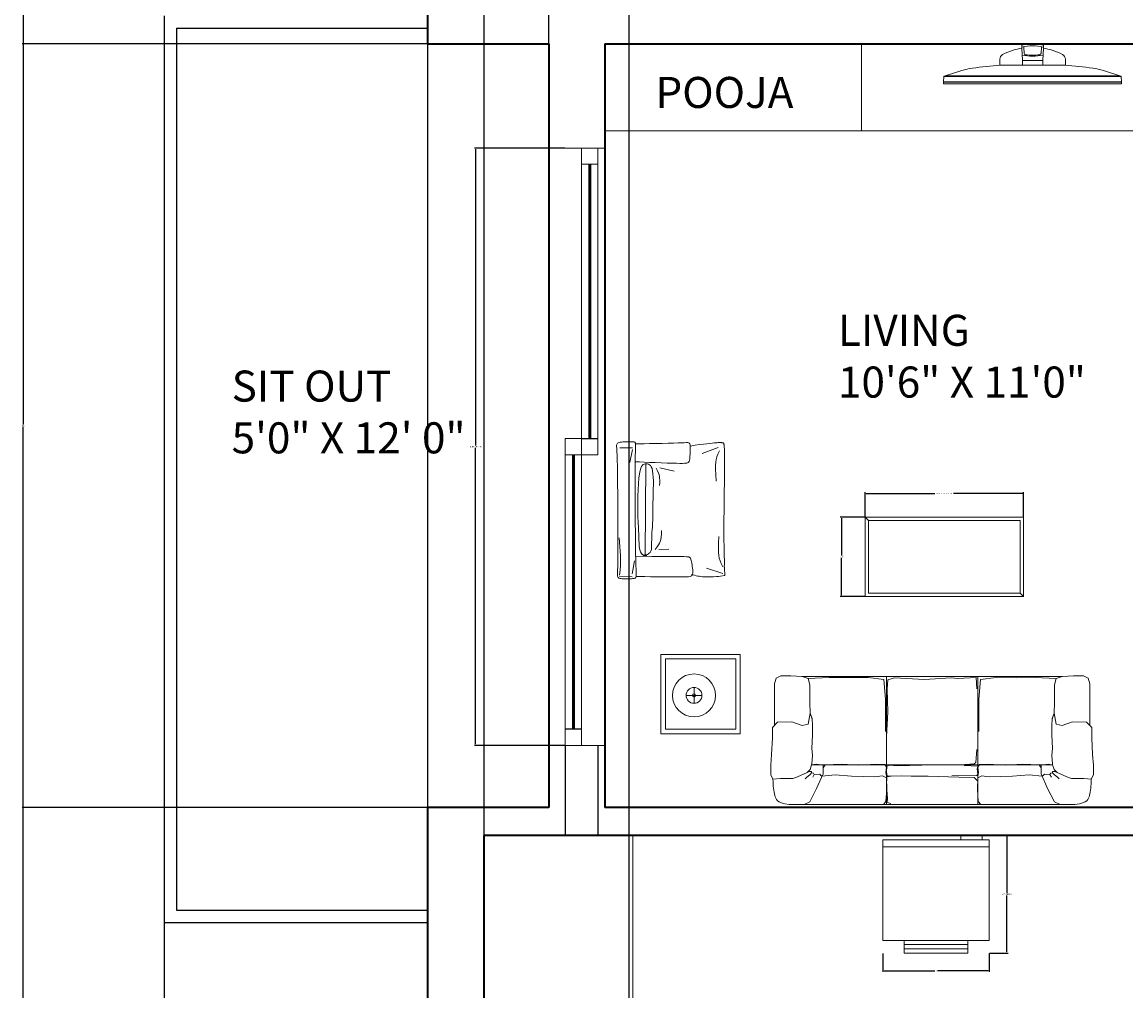
# Model space of a CAD drawing. Units: inches. Extents: x 1723 to 2209, y 1326 to 1810.
# Tile 2 of 6: x 1723 to 1901, y 1477 to 1633. Entities that reach past the tile are written whole.
import ezdxf

# ---------------------------------------------------------------- set-up
doc = ezdxf.new("R2010")
doc.units = ezdxf.units.IN
doc.layers.get('Defpoints').update_dxf_attribs({"color": 255})
for name, color, linetype, lineweight in [('A-ANNO-DIMS', 2, 'Continuous', 18), ('A-AREA-IDEN', 7, 'Continuous', 18), ('A-EQPM', 8, 'Continuous', 13), ('A-FLOR', 7, 'Continuous', 25), ('A-FLOR-CASE', 9, 'Continuous', 18), ('A-FURN', 8, 'Continuous', 13), ('A-WALL', 7, 'Continuous', 35), ('Sliding Door', 3, 'Continuous', 18)]:
    doc.layers.add(name, color=color, linetype=linetype, lineweight=lineweight)
doc.styles.get("Standard").update_dxf_attribs({"font": 'arial.ttf'})
doc.dimstyles.get("Standard").update_dxf_attribs({"dimtxt": 0.18, "dimasz": 0.18, "dimexe": 0.18, "dimexo": 0.0625, "dimgap": 0.09, "dimtad": 0, "dimtih": 1, "dimtoh": 1, "dimdec": 4, "dimzin": 0, "dimdsep": 46, "dimtxsty": 'Standard', "dimcen": 0.09, "dimadec": 0, "dimazin": 0, "dimtfac": 1, "dimtdec": 4, "dimtofl": 0, "dimtmove": 0, "dimatfit": 3, "dimfxl": 1, "dimtolj": 1, "dimtzin": 0, "dimarcsym": 0})

# ---------------------------------------------------------------- blocks, each defined once
blk = doc.blocks.new('A$C15BA614B')
for p, q in [((0, 720), (0, 81)), ((675, 720), (0, 720)), ((495, 747), (495, 720)), ((630, 747), (495, 747)), ((630, 720), (630, 747)), ((675, 81), (675, 720)), ((675, 675), (0, 675)), ((0, 81), (675, 81)), ((135, 81), (135, 0)), ((540, 81), (540, 0)), ((135, 54), (540, 54)), ((135, 27), (540, 27)), ((135, 0), (540, 0))]:
    blk.add_line(p, q)
blk = doc.blocks.new('sofa 053')
at = {"color": 0}
for p, q in [((-919.5, 900), (188.2, 900)), ((-325.8, 0), (-325.8, 900)), ((-317.6, 813.6), (-313, 892.1)), ((-185.2, 885.5), (-313, 892.1)), ((-185.2, 885.5), (-139.6, 891.1)), ((-139.6, 891.1), (48.6, 880)), ((48.6, 880), (260.2, 891.1)), ((188.2, 900), (316.6, 900)), ((260.2, 891.1), (305.9, 877.2)), ((305.9, 877.2), (311.4, 812.2)), ((316.6, 0), (316.6, 900)), ((316.6, 900), (316.6, 0)), ((910.3, 900), (316.6, 900)), ((311.4, 812.2), (305.9, 651.8)), ((305.9, 651.8), (316.6, 476.9)), ((-850.9, 280), (188.2, 280)), ((188.2, 280), (316.6, 280)), ((841.8, 280), (316.6, 280)), ((143.1, 200.9), (209.4, 202.3)), ((209.4, 202.3), (282.4, 200.9)), ((-997.7, 0), (188.2, 0)), ((188.2, 0), (316.6, 0)), ((988.6, 0), (316.6, 0))]:
    blk.add_line(p, q, dxfattribs=at)
for points in [[(-1112.2, 556.2), (-1112.6, 849.1), (-1101.3, 888.6), (-1067.5, 905.5), (-996.9, 905.5), (-917.9, 899.9), (-875.6, 885.8), (-864.3, 840.7), (-864.3, 716.5), (-861.8, 642.8)], [(-875.6, 885.8), (-728.9, 894.2)], [(-598.4, 891.4), (-454.5, 894.2), (-344.5, 880.1), (-333.2, 741.9), (-333.2, 513.4)], [(719.7, 894.2), (445.3, 894.2), (335.3, 880.1), (324, 741.9), (324, 513.4)], [(866.4, 885.8), (719.7, 894.2)], [(1103, 556.2), (1103.5, 849.1), (1092.2, 888.6), (1058.3, 905.5), (987.8, 905.5), (908.8, 899.9), (866.4, 885.8), (855.1, 840.7), (855.1, 716.5), (852.6, 642.8)], [(-983, 183.4), (-1070.3, 183.4), (-1122.9, 178.4), (-1138, 208.8), (-1138, 276.5), (-1132.4, 352.7), (-1126.7, 468.3), (-1126.7, 541.7), (-1090.1, 578.3), (-991.3, 581.1), (-917.9, 555.8), (-875.6, 564.2), (-861.8, 642.8), (-861.8, 642.8), (-847.2, 601.3)], [(-861.8, 642.8), (-847.4, 605.8), (-845.2, 554.1), (-845.2, 488.4), (-849.5, 396.9), (-845.2, 345.2), (-849.5, 285.9), (-850.9, 280)], [(852.6, 642.8), (838.2, 605.8), (836, 554.1), (836, 488.4), (840.3, 396.9), (836, 345.2), (840.3, 285.9), (841.8, 280)], [(973.8, 183.4), (1061.1, 183.4), (1113.7, 178.4), (1128.9, 208.8), (1128.9, 276.5), (1123.2, 352.7), (1117.6, 468.3), (1117.6, 541.7), (1080.9, 578.3), (982.1, 581.1), (908.8, 555.8), (866.4, 564.2), (852.6, 642.8), (852.6, 642.8), (838, 601.3)], [(-317.8, 387.7), (-312.2, 296.4), (-299.8, 286.8), (-201.6, 279.8)], [(-850.9, 280), (-861.2, 247.6), (-882.3, 226.5), (-951.2, 195.1), (-983, 183.4)], [(-850.9, 280), (-819.2, 285), (-771.2, 276.5), (-771.2, 217.3), (-816.3, 112.9), (-864.3, 19.8), (-904, 0)], [(-771.2, 258.8), (-757.1, 279.3), (-639.4, 285.3), (-522.2, 277.6), (-394.4, 284.5), (-336.6, 281.4), (-325.9, 262.4), (-330.5, 225.2), (-325.8, 200)], [(-142.1, 202.3), (-318.5, 205.1), (-326.1, 214.9), (-321.9, 250.4), (-325.4, 270.6), (-229.9, 275.5)], [(67.1, 276.9), (241.3, 272), (295, 278.3), (313.1, 269.2), (315.9, 229.5), (310.3, 202.3), (282.4, 200.9), (313.8, 195.4), (316.6, 133.3), (309.6, 42.1), (311.7, 18.4), (285.9, 5.1)], [(762, 258.8), (747.9, 279.3), (630.3, 285.3), (513.1, 277.6), (385.3, 284.5), (327.4, 281.4), (316.8, 262.4), (321.3, 225.2), (316.6, 200)], [(841.8, 280), (810, 285), (762, 276.5), (762, 217.3), (807.2, 112.9), (855.1, 19.8), (894.8, 0)], [(841.8, 280), (852.1, 247.6), (873.1, 226.5), (942, 195.1), (973.8, 183.4)], [(-997.7, 0), (-1008.3, 1), (-1039.1, 5.9), (-1062.3, 11.8), (-1079.1, 18.7), (-1090.8, 26.4), (-1098.5, 35), (-1103.5, 44.4), (-1107, 54.4), (-1110, 65), (-1112.8, 76.3), (-1115.2, 88.2), (-1117.4, 101), (-1119.2, 114.6), (-1120.7, 129), (-1121.8, 144.4), (-1122.5, 160.9), (-1122.9, 178.4)], [(-882.3, 226.5), (-866.4, 231.7), (-851, 231.7), (-851, 222.6), (-862.2, 212.1), (-886.8, 189.7), (-897.3, 182)], [(-851, 222.6), (-838.4, 221.9), (-832.8, 211.4), (-842.6, 191.8)], [(-832.8, 211.4), (-793.6, 214.2), (-788, 206.5), (-778.7, 200)], [(-778.7, 200), (-686.5, 208.8), (-569.8, 200), (-406.1, 194.5), (-354.2, 201.3), (-325.2, 189.4), (-323.5, 107.7), (-328.6, 20.9), (-346.5, 0.5)], [(-323.7, 167.8), (-300.7, 189.7), (-191.3, 193), (24.3, 200.7), (143.1, 200.9)], [(769.5, 200), (677.4, 208.8), (560.7, 200), (396.9, 194.5), (345, 201.3), (316.1, 189.4), (314.3, 107.7), (319.5, 20.9), (337.3, 0.5)], [(823.7, 211.4), (784.4, 214.2), (778.8, 206.5), (769.5, 200)], [(841.9, 222.6), (829.3, 221.9), (823.7, 211.4), (833.5, 191.8)], [(873.1, 226.5), (857.3, 231.7), (841.9, 231.7), (841.9, 222.6), (853.1, 212.1), (877.6, 189.7), (888.1, 182)], [(988.6, 0), (999.2, 1), (1030, 5.9), (1053.2, 11.8), (1070, 18.7), (1081.6, 26.4), (1089.3, 35), (1094.3, 44.4), (1097.8, 54.4), (1100.9, 65), (1103.6, 76.3), (1106.1, 88.2), (1108.2, 101), (1110, 114.6), (1111.5, 129), (1112.6, 144.4), (1113.3, 160.9), (1113.7, 178.4)]]:
    blk.add_lwpolyline(points, dxfattribs=at)
at = {"color": 0, "flags": 128}
blk.add_lwpolyline([(-728.9, 894.2), (-598.4, 891.4)], dxfattribs=at)
blk = doc.blocks.new('armchair 042')
at = {"color": 0}
for p, q in [((672.7, 1002.5), (673.1, 1009.6)), ((673.1, 1009.6), (673.7, 1013.9)), ((673.7, 1013.9), (674.6, 1017.2)), ((674.6, 1017.2), (675.9, 1020.1)), ((675.9, 1020.1), (677.7, 1022.5)), ((677.7, 1022.5), (680.2, 1024.5)), ((680.2, 1024.5), (683.6, 1026.2)), ((683.6, 1026.2), (688, 1027.5)), ((688, 1027.5), (693.6, 1028.5)), ((693.6, 1028.5), (700.5, 1029.3)), ((700.5, 1029.3), (708.8, 1030)), ((708.8, 1030), (718.2, 1030.4)), ((718.2, 1030.4), (728.4, 1030.7)), ((728.4, 1030.7), (739, 1030.8)), ((739, 1030.8), (749.7, 1030.7)), ((749.7, 1030.7), (760.2, 1030.5)), ((760.2, 1030.5), (770.1, 1030.1)), ((770.1, 1030.1), (779, 1029.6)), ((779, 1029.6), (786.6, 1028.9)), ((786.6, 1028.9), (793.1, 1028)), ((793.1, 1028), (798.5, 1026.7)), ((798.5, 1026.7), (802.9, 1024.9)), ((802.9, 1024.9), (806.4, 1022.6)), ((806.4, 1022.6), (809.2, 1019.5)), ((809.2, 1019.5), (811.3, 1015.7)), ((811.3, 1015.7), (812.8, 1010.9)), ((812.8, 1010.9), (813.9, 1004.9)), ((813.9, 1004.9), (814.6, 996.9)), ((672.5, 990.1), (672.7, 1002.5)), ((672.5, 984.9), (672.5, 990.1)), ((677.3, 823.2), (672.5, 984.9)), ((814.6, 996.9), (812.5, 908.4)), ((573.7, 837.2), (567.5, 829.9)), ((580.3, 842.4), (573.7, 837.2)), ((587.4, 846), (580.3, 842.4)), ((594.9, 848.2), (587.4, 846)), ((599.1, 854), (591.5, 852.6)), ((602.5, 849.6), (594.9, 848.2)), ((606.8, 854.5), (599.1, 854)), ((610.2, 850.1), (602.5, 849.6)), ((614.4, 853.6), (606.8, 854.5)), ((617.8, 849.1), (610.2, 850.1)), ((621.8, 850), (614.4, 853.6)), ((625.2, 845.6), (617.8, 849.1)), ((628.9, 843), (621.8, 850)), ((632.3, 838.5), (625.2, 845.6)), ((638.8, 826.9), (632.3, 838.5)), ((812.5, 908.4), (812.4, 826.8)), ((557.4, 807.7), (553.9, 678.4)), ((562.1, 820.2), (557.4, 807.7)), ((567.5, 829.9), (562.1, 820.2)), ((644.7, 809.8), (638.8, 826.9)), ((649.7, 786.2), (644.7, 809.8)), ((649.7, 786.2), (654.1, 641.6)), ((678.2, 701.5), (677.3, 823.2)), ((812.4, 826.8), (811.1, 761.6)), ((811.1, 761.6), (811.2, 680.2)), ((7.4, 656), (7.5, 675.3)), ((7.5, 675.3), (7.6, 690.1)), ((7.6, 690.1), (7.8, 709)), ((7.8, 709), (7.9, 714.5)), ((7.9, 714.5), (8, 718.1)), ((553.9, 678.4), (551.1, 659.3)), ((679, 583.6), (678.2, 701.5)), ((811.2, 680.2), (811.3, 600.4)), ((6.9, 566.8), (7.1, 601.6)), ((7.1, 601.6), (7.3, 631.6)), ((7.3, 631.6), (7.4, 656)), ((547.8, 611.8), (547, 584.1)), ((549.1, 637), (547.8, 611.8)), ((551.1, 659.3), (549.1, 637)), ((657.1, 602.6), (654.1, 641.6)), ((659, 557.1), (657.1, 602.6)), ((811.3, 600.4), (811.6, 523.4)), ((4.6, 404), (6.7, 527.8)), ((6.7, 527.8), (6.9, 566.8)), ((546.2, 522.8), (545.8, 489.8)), ((546.5, 554.3), (546.2, 522.8)), ((547, 584.1), (546.5, 554.3)), ((660, 507.3), (659, 557.1)), ((660, 455.3), (660, 507.3)), ((679.6, 474.1), (679, 583.6)), ((811.6, 523.4), (811.9, 450)), ((544.6, 421.1), (543.6, 386.4)), ((545.3, 455.8), (544.6, 421.1)), ((545.8, 489.8), (545.3, 455.8)), ((659, 403.2), (660, 455.3)), ((680.1, 377.5), (679.6, 474.1)), ((811.9, 450), (812.4, 381.2)), ((4.3, 316.1), (4.4, 359.1)), ((4.4, 359.1), (4.6, 404)), ((542.8, 352.2), (542.3, 319.3)), ((543.6, 386.4), (542.8, 352.2)), ((654.7, 307), (657.3, 353.1)), ((657.3, 353.1), (659, 403.2)), ((680.4, 297.5), (680.1, 377.5)), ((812.4, 381.2), (812.9, 318)), ((4, 237.4), (4.1, 275.4)), ((4.1, 275.4), (4.3, 316.1)), ((542.3, 319.3), (542.4, 288.3)), ((542.4, 288.3), (543.2, 259.8)), ((543.2, 259.8), (545, 234.5)), ((647.4, 234.9), (651.4, 267.1)), ((651.4, 267.1), (654.7, 307)), ((680.4, 233), (680.4, 297.5)), ((812.9, 318), (813.5, 261.3)), ((813.5, 261.3), (814.1, 212)), ((3.7, 145), (3.8, 171.8)), ((3.8, 171.8), (3.9, 202.7)), ((3.9, 202.7), (4, 237.4)), ((545, 234.5), (548, 213)), ((548, 213), (552.3, 195.8)), ((552.3, 195.8), (557.9, 182.6)), ((557.9, 182.6), (564.4, 172.9)), ((564.4, 172.9), (571.6, 166.2)), ((618.7, 164), (625.5, 169.4)), ((625.5, 169.4), (631.8, 178.2)), ((631.8, 178.2), (637.6, 191.4)), ((637.6, 191.4), (642.8, 210)), ((642.8, 210), (647.4, 234.9)), ((680.1, 142.7), (680.3, 182.1)), ((680.3, 182.1), (680.4, 233)), ((814.1, 212), (814.8, 170.8)), ((814.8, 170.8), (815.5, 137.1)), ((3.6, 122.8), (3.7, 145)), ((3.6, 104.6), (3.6, 122.8)), ((3.6, 89.9), (3.6, 104.6)), ((3.6, 78.1), (3.6, 89.9)), ((571.6, 166.2), (579.4, 162.1)), ((579.4, 162.1), (587.5, 159.9)), ((587.5, 159.9), (595.7, 159.4)), ((595.7, 159.4), (603.7, 159.9)), ((603.7, 159.9), (611.4, 161.2)), ((611.4, 161.2), (618.7, 164)), ((678.8, 73.3), (679.3, 90.3)), ((679.3, 90.3), (679.7, 112.7)), ((679.7, 112.7), (680.1, 142.7)), ((815.5, 137.1), (816.3, 109.9)), ((816.3, 109.9), (817.1, 88.3)), ((817.1, 88.3), (817.8, 71.3)), ((3.6, 68.7), (3.6, 78.1)), ((3.7, 61), (3.6, 68.7)), ((3.9, 54.4), (3.7, 61)), ((4.1, 48.4), (3.9, 54.4)), ((4.3, 42.5), (4.1, 48.4)), ((4.6, 36.7), (4.3, 42.5)), ((5, 31), (4.6, 36.7)), ((5.4, 25.6), (5, 31)), ((5.9, 20.6), (5.4, 25.6)), ((6.4, 16.1), (5.9, 20.6)), ((6.9, 12.1), (6.4, 16.1)), ((7.5, 8.7), (6.9, 12.1)), ((8.1, 6.1), (7.5, 8.7)), ((8.7, 4.2), (8.1, 6.1)), ((9.4, 2.8), (8.7, 4.2)), ((10.1, 1.9), (9.4, 2.8)), ((10.9, 1.3), (10.1, 1.9)), ((11.8, 1), (10.9, 1.3)), ((12.7, 0.8), (11.8, 1)), ((13.8, 0.7), (12.7, 0.8)), ((15, 0.5), (13.8, 0.7)), ((16.4, 0.2), (15, 0.5)), ((17.8, 0), (16.4, 0.2)), ((69.7, 0.1), (59.3, -0.6)), ((82.4, 1.2), (69.7, 0.1)), ((97.7, 2.6), (82.4, 1.2)), ((115.9, 4.5), (97.7, 2.6)), ((137.4, 6.9), (115.9, 4.5)), ((162.6, 10), (137.4, 6.9)), ((191.8, 13.8), (162.6, 10)), ((225.3, 18.6), (191.8, 13.8)), ((263.5, 24.3), (225.3, 18.6)), ((676.8, 20.1), (676.9, 28.1)), ((676.9, 13.3), (676.8, 20.1)), ((676.9, 28.1), (677.3, 37.3)), ((677.3, 7.6), (676.9, 13.3)), ((677.3, 37.3), (677.7, 47.8)), ((678.1, 3), (677.3, 7.6)), ((677.7, 47.8), (678.2, 59.7)), ((679.4, -0.7), (678.1, 3)), ((678.2, 59.7), (678.8, 73.3)), ((796.6, 38.6), (701.3, 38)), ((813.7, 3.1), (808.9, -0.2)), ((817.1, 7.1), (813.7, 3.1)), ((819.2, 11.8), (817.1, 7.1)), ((817.8, 71.3), (818.6, 58)), ((818.6, 58), (819.2, 47.4)), ((819.2, 47.4), (819.9, 38.5)), ((820.3, 17.3), (819.2, 11.8)), ((819.9, 38.5), (820.4, 30.7)), ((820.6, 23.6), (820.3, 17.3)), ((820.4, 30.7), (820.6, 23.6)), ((19.4, -0.3), (17.8, 0)), ((21, -0.6), (19.4, -0.3)), ((22.8, -0.9), (21, -0.6)), ((24.7, -1.2), (22.8, -0.9)), ((26.7, -1.4), (24.7, -1.2)), ((28.9, -1.7), (26.7, -1.4)), ((31.5, -1.8), (28.9, -1.7)), ((34.7, -1.9), (31.5, -1.8)), ((38.8, -1.8), (34.7, -1.9)), ((44.1, -1.6), (38.8, -1.8)), ((50.8, -1.2), (44.1, -1.6)), ((59.3, -0.6), (50.8, -1.2)), ((681.2, -3.5), (679.4, -0.7)), ((683.6, -5.5), (681.2, -3.5)), ((686.7, -6.8), (683.6, -5.5)), ((690.7, -7.5), (686.7, -6.8)), ((695.7, -7.9), (690.7, -7.5)), ((701.7, -8), (695.7, -7.9)), ((709, -7.9), (701.7, -8)), ((717.6, -7.9), (709, -7.9)), ((727.6, -7.9), (717.6, -7.9)), ((738.6, -7.9), (727.6, -7.9)), ((750.2, -7.8), (738.6, -7.9)), ((761.9, -7.6), (750.2, -7.8)), ((773.5, -7.1), (761.9, -7.6)), ((784.4, -6.2), (773.5, -7.1)), ((794.2, -4.8), (784.4, -6.2)), ((802.5, -2.8), (794.2, -4.8)), ((808.9, -0.2), (802.5, -2.8))]:
    blk.add_line(p, q, dxfattribs=at)
for points in [[(673.7, 1013.8), (664.2, 1013.8), (640.7, 1014), (606.1, 1014.2), (563.7, 1014.5), (516.6, 1014.8), (467.8, 1015.2), (420.6, 1015.6), (378, 1016), (342.6, 1016.4), (314.1, 1016.4), (291.8, 1016), (274.9, 1014.7), (262.6, 1012.3), (254.1, 1008.5), (248.7, 1003), (245.5, 995.6), (243.8, 986.1), (243.3, 974.9), (243.8, 962.5), (245.1, 949.4), (247, 936.2), (249.2, 923.3), (251.5, 911.2), (253.7, 900.6), (255.7, 891.7), (257.5, 884.5), (259.4, 878.8), (261.4, 874.3), (263.7, 870.9), (266.5, 868.4), (270, 866.5), (274.3, 865), (280.2, 863.8), (291, 862.8), (310.5, 862.1), (342.6, 861.7), (391.2, 861.7), (460.2, 861.9), (553.4, 862.5), (673.3, 863.5)], [(703.5, 1015.3), (798.9, 1012.7)], [(15.9, 939.3), (27.9, 914.2), (36.8, 893.4), (43.1, 874.3), (47.1, 854.2), (49.1, 830.5), (49.5, 800.4), (48.8, 761.3), (47.1, 710.5)], [(16.5, 991), (139.2, 949.8)], [(684.9, 894.8), (703.3, 993.6)], [(799.2, 1003.9), (794.7, 964.3), (792.3, 926.3), (791.7, 889.9), (792.5, 854.6), (794.2, 820.3), (796.4, 786.7), (798.9, 753.6), (801.1, 720.8)], [(600.2, 159.7), (604.6, 849.6)], [(501.8, 809.3), (426, 805)], [(528.6, 807.4), (514.3, 788.5), (503.5, 773.2), (495.6, 759.9), (490, 746.9), (486.2, 732.5), (483.5, 715.1), (481.5, 693), (479.5, 664.4)], [(41.4, 59.9), (52.5, 85.4), (60.8, 106.5), (66.4, 125.8), (69.7, 146), (71, 169.8), (70.4, 199.8), (68.3, 238.9), (65, 289.7)], [(520, 190.9), (510.9, 212.2), (504.2, 229), (499.4, 243), (496.2, 255.5), (494.5, 268.3), (493.9, 282.7), (494, 300.5), (494.7, 323.1)], [(493, 189.5), (383.5, 215.7)], [(677.3, 8), (668.7, 7.9), (645.8, 7.5), (611.9, 6.9), (570.2, 6.1), (523.8, 5.2), (476, 4.2), (429.9, 3.1), (388.9, 2), (355.3, 0.9), (328.9, 0), (308.8, -0.8), (294, -1.3), (283.6, -1.4), (276.7, -0.9), (272.3, 0), (269.4, 1.7), (267.3, 4.1), (265.7, 7.3), (264.6, 11.3), (263.9, 16.1), (263.5, 21.6), (263.3, 28), (263.3, 35.2), (263.3, 43.1), (263.4, 51.8), (263.6, 61.2), (263.7, 70.8), (263.9, 80.6), (264.2, 90.2), (264.6, 99.5), (265, 108.3), (265.6, 116.2), (266.3, 123.1), (267.2, 129.1), (268.2, 134.2), (269.6, 138.5), (271.3, 142.2), (273.5, 145.3), (276, 147.8), (279.1, 150), (282.9, 151.8), (288.1, 153.3), (295.6, 154.4), (306.3, 155.2), (321.1, 155.6), (340.9, 155.6), (366.5, 155.1), (398.8, 154.3), (438, 153.1), (482, 151.5), (527.7, 149.8), (572.3, 148.1), (612.9, 146.4), (646.6, 145.1), (670.5, 144.1), (680, 143.7)], [(701.2, 49.6), (719.7, 148.3)], [(50.8, 35.6), (172, 80.9)]]:
    blk.add_lwpolyline(points, dxfattribs=at)
for centre, radius, start, end in [((4.2, 1001.7), 3.43, 101.07019, 170.34951), ((159.3, 182.2), 837.5, 96.59178, 100.71955), ((769.8, -30414.4), 31436.5, 91.11446, 91.28806), ((117.9, 570.8), 447.1, 72.48852, 84.80948), ((57, 992.7), 57, 170.34951, 189.46286), ((-256.2, 940.5), 260.5, 0.55092, 9.46286), ((4370.1, 901.7), 4365.9, 179.458, 182.40994)]:
    blk.add_arc(centre, radius, start, end, dxfattribs=at)
blk = doc.blocks.new('B1')
at = {"color": 0}
for points in [[(-73.6, -0.1), (-73.6, 13.1, -0.272026), (-67.3, 23.9, -0.059641), (-43.9, 33.5, -0.024069), (-24.5, 37.9), (-22.7, 10), (-22.7, 0)], [(-24.5, 37.9), (-24.5, 43.2, -0.236854), (-23.9, 44.5, -0.069077), (0, 47.8, -0.069077)], [(-24.5, 37.7), (-24.5, 38.9, -0.236854), (-23.9, 40.2, -0.069077), (0, 43.6, -0.069077)], [(24.5, 37.9), (24.5, 43.2, 0.236854), (23.9, 44.5, 0.069077), (0, 47.8, 0.069077)], [(24.5, 37.7), (24.5, 38.9, 0.236854), (23.9, 40.2, 0.069077), (0, 43.6, 0.069077)], [(73.6, -0.1), (73.6, 13.1, 0.272026), (67.3, 23.9, 0.059641), (43.9, 33.5, 0.024069), (24.5, 37.9), (22.7, 10), (22.7, 0)], [(-200, -38.4), (-200, -37.7), (-199.2, -25.8, -0.303983), (-198.5, -24.8), (-159.1, -12.4, -0.039649), (-135.4, -7, -0.017831), (-72.5, 0), (0, 0)], [(200, -38.4), (200, -37.7), (199.2, -25.8, 0.303983), (198.5, -24.8), (159.1, -12.4, 0.039649), (135.4, -7, 0.017831), (72.5, 0), (0, 0)]]:
    blk.add_lwpolyline(points, format="xyb", dxfattribs=at)
for points in [[(-19.8, 40.1), (-18.9, 26.4)], [(19.8, 40.1), (18.9, 26.4)], [(-22.7, 10), (0, 10)], [(22.7, 10), (0, 10)], [(-196.3, -24.2), (0, -24.2)], [(196.3, -24.2), (0, -24.2)], [(-200, -37.8), (0, -37.8)], [(-200, -41.4), (-200, -38.4), (200, -38.4)], [(-200, -38.4), (0, -38.4)], [(200, -41.4), (200, -38.4), (-200, -38.4)], [(-199.2, -25.8), (0, -25.8)], [(-198.9, -42.4), (0, -42.4)], [(199.2, -25.8), (0, -25.8)], [(200, -37.8), (0, -37.8)], [(200, -38.4), (0, -38.4)], [(198.9, -42.4), (0, -42.4)]]:
    blk.add_lwpolyline(points, dxfattribs=at)
for centre, radius, start, end in [((-15.4, 26.6), 3.53, 183.678, 262.9963), ((15.4, 26.6), 3.53, 277.0037, 356.322), ((0, 150), 130, 259.5789, 270), ((0, 152.2), 130, 262.9963, 270), ((0, 152.2), 130, 270, 277.0037), ((0, 150), 130, 270, 280.4211), ((-198.9, -41.4), 1.06, 180, 270), ((198.9, -41.4), 1.06, 270, 0)]:
    blk.add_arc(centre, radius, start, end, dxfattribs=at)
blk = doc.blocks.new('A$C7a76cbd6')
at = {"layer": 'Sliding Door'}
for p, q in [((540.4, 283.7, 0), (478.3, 283.7, 0)), ((478.3, 283.7, 0), (540.4, 283.7, 0)), ((540.4, 221.5, 0), (540.4, 283.7, 0)), ((540.4, 283.7, 0), (1585.3, 283.7, 0)), ((540.4, 283.7, 0), (540.4, 221.5, 0)), ((1585.3, 256.6, 0), (540.4, 256.6, 0)), ((540.4, 256.6, 0), (540.4, 248.7, 0)), ((540.4, 252.6, 0), (1584.3, 252.6, 0)), ((1584.3, 283.7, 0), (1647.4, 283.7, 0)), ((1584.3, 283.7, 0), (1584.3, 221.5, 0)), ((1647.4, 283.7, 0), (1585.3, 283.7, 0)), ((1585.3, 283.7, 0), (1585.3, 221.5, 0)), ((1585.3, 248.7, 0), (1585.3, 256.6, 0)), ((1647.4, 221.5, 0), (1647.4, 283.7, 0)), ((1647.4, 283.7, 0), (1647.4, 221.5, 0)), ((478.3, 221.5, 0), (540.4, 221.5, 0)), ((478.3, 221.5, 0), (540.4, 221.5, 0)), ((540.4, 248.7, 0), (1585.3, 248.7, 0)), ((1584.3, 221.5, 0), (540.4, 221.5, 0)), ((1646.4, 221.5, 0), (1584.3, 221.5, 0)), ((1584.3, 221.5, 0), (1584.3, 159.4, 0)), ((1584.3, 221.5, 0), (1647.4, 221.5, 0)), ((1584.3, 221.5, 0), (1647.4, 221.5, 0)), ((1584.3, 221.5, 0), (1584.3, 159.4, 0)), ((1585.3, 221.5, 0), (1647.4, 221.5, 0)), ((1646.4, 159.4, 0), (1646.4, 221.5, 0)), ((1647.4, 221.5, 0), (2691.3, 221.5, 0)), ((1647.4, 221.5, 0), (1647.4, 159.4, 0)), ((2690.3, 221.5, 0), (2753.4, 221.5, 0)), ((2690.3, 221.5, 0), (2690.3, 159.4, 0)), ((2753.4, 221.5, 0), (2691.3, 221.5, 0)), ((2691.3, 221.5, 0), (2691.3, 159.4, 0)), ((2691.3, 194.4, 0), (1647.4, 194.4, 0)), ((1647.4, 194.4, 0), (1647.4, 186.5, 0)), ((1647.4, 190.5, 0), (2690.3, 190.5, 0)), ((1647.4, 186.5, 0), (2691.3, 186.5, 0)), ((2691.3, 186.5, 0), (2691.3, 194.4, 0)), ((1584.3, 159.4, 0), (1646.4, 159.4, 0)), ((1584.3, 159.4, 0), (1647.4, 159.4, 0)), ((2691.3, 159.4, 0), (1646.4, 159.4, 0)), ((2690.3, 159.4, 0), (2753.4, 159.4, 0)), ((2691.3, 159.4, 0), (2753.4, 159.4, 0))]:
    blk.add_line(p, q, dxfattribs=at)
blk = doc.blocks.new('TABLE-END-SMALL')
for p, q in [((5.32, 4.88), (5.32, 7.45)), ((6.6, 6.17), (4.03, 6.17))]:
    blk.add_line(p, q)
for points in [[(0, 0), (12.75, 0), (12.75, 12.75), (0, 12.75)], [(0.71, 0.71), (12.04, 0.71), (12.04, 12.04), (0.71, 12.04)]]:
    blk.add_lwpolyline(points, close=True)
for radius in [3.46, 1.28, 0.266]:
    blk.add_circle((5.32, 6.17), radius)
blk = doc.blocks.new('TABLE-COFFEE-RECT')
for p, q in [((0, 0), (0, 12.75)), ((0, 12.75), (0.53, 12.22)), ((0, 12.75), (25.5, 12.75)), ((25.5, 12.75), (25.5, 0)), ((0.53, 0.53), (0.53, 12.22)), ((0.53, 12.22), (24.97, 12.22)), ((24.97, 12.22), (24.97, 0.53)), ((25.5, 0), (0, 0)), ((24.97, 0.53), (0.53, 0.53)), ((24.97, 0.53), (25.5, 0))]:
    blk.add_line(p, q)
blk = doc.blocks.new('*D63')
at = {"layer": 'A-ANNO-DIMS', "color": 0, "lineweight": -2, "transparency": 16777216}
for p, q in [((1810.16, 1612.41), (1795.61, 1612.41)), ((1795.79, 1612.23), (1795.79, 1564.49)), ((1795.79, 1516.38), (1795.79, 1564.12)), ((1810.16, 1516.2), (1795.61, 1516.2))]:
    blk.add_line(p, q, dxfattribs=at)
at = {"layer": 'A-ANNO-DIMS', "color": 0, "transparency": 16777216}
for points in [[(1795.76, 1612.23), (1795.82, 1612.23), (1795.79, 1612.41)], [(1795.76, 1516.38), (1795.82, 1516.38), (1795.79, 1516.2)]]:
    blk.add_solid(points, dxfattribs=at)
at = {"layer": 'Defpoints', "color": 0, "transparency": 16777216}
for p in [(1810.22, 1612.41), (1795.79, 1516.2), (1810.22, 1516.2)]:
    blk.add_point(p, dxfattribs=at)
at = {"layer": 'A-ANNO-DIMS', "color": 0, "transparency": 16777216, "insert": (1795.79, 1564.31), "char_height": 0.18, "attachment_point": 5}
blk.add_mtext('\\A1;SLIDING UNIT 96', dxfattribs=at)
blk = doc.blocks.new('*D64')
at = {"layer": 'A-ANNO-DIMS', "color": 0, "lineweight": -2, "transparency": 16777216}
for p, q in [((1810.22, 1516.14), (1810.22, 1501.59)), ((1815.48, 1516.14), (1815.48, 1501.59)), ((1810.4, 1501.77), (1812.7, 1501.77)), ((1815.3, 1501.77), (1813, 1501.77))]:
    blk.add_line(p, q, dxfattribs=at)
at = {"layer": 'A-ANNO-DIMS', "color": 0, "transparency": 16777216}
for points in [[(1810.4, 1501.8), (1810.4, 1501.74), (1810.22, 1501.77)], [(1815.3, 1501.8), (1815.3, 1501.74), (1815.48, 1501.77)]]:
    blk.add_solid(points, dxfattribs=at)
at = {"layer": 'Defpoints', "color": 0, "transparency": 16777216}
for p in [(1810.22, 1516.2), (1815.48, 1516.2), (1815.48, 1501.77)]:
    blk.add_point(p, dxfattribs=at)
at = {"layer": 'A-ANNO-DIMS', "color": 0, "transparency": 16777216, "insert": (1812.85, 1501.77), "char_height": 0.18, "attachment_point": 5}
blk.add_mtext('\\A1;5', dxfattribs=at)
blk = doc.blocks.new('*D75')
at = {"layer": 'A-ANNO-DIMS', "color": 0, "lineweight": -2, "transparency": 16777216}
for p, q in [((1858.52, 1553.01), (1858.52, 1556.96)), ((1858.7, 1556.78), (1869.77, 1556.78)), ((1883.85, 1556.78), (1872.78, 1556.78)), ((1884.03, 1553.01), (1884.03, 1556.96))]:
    blk.add_line(p, q, dxfattribs=at)
at = {"layer": 'A-ANNO-DIMS', "color": 0, "transparency": 16777216}
for points in [[(1858.7, 1556.81), (1858.7, 1556.75), (1858.52, 1556.78)], [(1883.85, 1556.81), (1883.85, 1556.75), (1884.03, 1556.78)]]:
    blk.add_solid(points, dxfattribs=at)
at = {"layer": 'Defpoints', "color": 0, "transparency": 16777216}
for p in [(1858.52, 1556.78), (1858.52, 1552.95), (1884.03, 1552.95)]:
    blk.add_point(p, dxfattribs=at)
at = {"layer": 'A-ANNO-DIMS', "color": 0, "transparency": 16777216, "insert": (1871.28, 1556.78), "char_height": 0.18, "attachment_point": 5}
blk.add_mtext('\\A1;COFFEE TABLE 26 TYP.', dxfattribs=at)
blk = doc.blocks.new('*D76')
at = {"layer": 'A-ANNO-DIMS', "color": 0, "lineweight": -2, "transparency": 16777216}
for p, q in [((1858.46, 1552.95), (1854.52, 1552.95)), ((1854.7, 1552.77), (1854.7, 1546.76)), ((1854.7, 1540.38), (1854.7, 1546.39)), ((1858.46, 1540.2), (1854.52, 1540.2))]:
    blk.add_line(p, q, dxfattribs=at)
at = {"layer": 'A-ANNO-DIMS', "color": 0, "transparency": 16777216}
for points in [[(1854.67, 1552.77), (1854.73, 1552.77), (1854.7, 1552.95)], [(1854.67, 1540.38), (1854.73, 1540.38), (1854.7, 1540.2)]]:
    blk.add_solid(points, dxfattribs=at)
at = {"layer": 'Defpoints', "color": 0, "transparency": 16777216}
for p in [(1858.52, 1552.95), (1854.7, 1540.2), (1858.52, 1540.2)]:
    blk.add_point(p, dxfattribs=at)
at = {"layer": 'A-ANNO-DIMS', "color": 0, "transparency": 16777216, "insert": (1854.7, 1546.57), "char_height": 0.18, "attachment_point": 5}
blk.add_mtext('\\A1;13 TYP.', dxfattribs=at)
blk = doc.blocks.new('*D87')
at = {"layer": 'A-ANNO-DIMS', "color": 0, "lineweight": -2, "transparency": 16777216}
for p, q in [((1878.58, 1501.69), (1881.54, 1501.69)), ((1881.36, 1501.51), (1881.36, 1492.4)), ((1881.36, 1482.93), (1881.36, 1492.04)), ((1878.58, 1482.75), (1881.54, 1482.75))]:
    blk.add_line(p, q, dxfattribs=at)
at = {"layer": 'A-ANNO-DIMS', "color": 0, "transparency": 16777216}
for points in [[(1881.33, 1501.51), (1881.39, 1501.51), (1881.36, 1501.69)], [(1881.33, 1482.93), (1881.39, 1482.93), (1881.36, 1482.75)]]:
    blk.add_solid(points, dxfattribs=at)
at = {"layer": 'Defpoints', "color": 0, "transparency": 16777216}
for p in [(1878.52, 1501.69), (1881.36, 1501.69), (1878.52, 1482.75)]:
    blk.add_point(p, dxfattribs=at)
at = {"layer": 'A-ANNO-DIMS', "color": 0, "transparency": 16777216, "insert": (1881.36, 1492.22), "char_height": 0.18, "attachment_point": 5}
blk.add_mtext('\\A1;APPLIANCE 19', dxfattribs=at)
blk = doc.blocks.new('*D88')
at = {"layer": 'A-ANNO-DIMS', "color": 0, "lineweight": -2, "transparency": 16777216}
for p, q in [((1861.4, 1482.69), (1861.4, 1479.73)), ((1878.52, 1482.69), (1878.52, 1479.73)), ((1861.58, 1479.91), (1869.75, 1479.91)), ((1878.34, 1479.91), (1870.17, 1479.91))]:
    blk.add_line(p, q, dxfattribs=at)
at = {"layer": 'A-ANNO-DIMS', "color": 0, "transparency": 16777216}
for points in [[(1861.58, 1479.94), (1861.58, 1479.88), (1861.4, 1479.91)], [(1878.34, 1479.94), (1878.34, 1479.88), (1878.52, 1479.91)]]:
    blk.add_solid(points, dxfattribs=at)
at = {"layer": 'Defpoints', "color": 0, "transparency": 16777216}
for p in [(1861.4, 1482.75), (1878.52, 1482.75), (1878.52, 1479.91)]:
    blk.add_point(p, dxfattribs=at)
at = {"layer": 'A-ANNO-DIMS', "color": 0, "transparency": 16777216, "insert": (1869.96, 1479.91), "char_height": 0.18, "attachment_point": 5}
blk.add_mtext('\\A1;17', dxfattribs=at)
blk = doc.blocks.new('*D94')
at = {"layer": 'A-ANNO-DIMS', "color": 0, "lineweight": -2, "transparency": 16777216}
for p, q in [((1788.04, 1786.69), (1722.75, 1786.69)), ((1722.93, 1786.51), (1722.93, 1567.87)), ((1722.93, 1348.87), (1722.93, 1567.51)), ((1788.04, 1348.69), (1722.75, 1348.69))]:
    blk.add_line(p, q, dxfattribs=at)
at = {"layer": 'A-ANNO-DIMS', "color": 0, "transparency": 16777216}
for points in [[(1722.9, 1786.51), (1722.96, 1786.51), (1722.93, 1786.69)], [(1722.9, 1348.87), (1722.96, 1348.87), (1722.93, 1348.69)]]:
    blk.add_solid(points, dxfattribs=at)
at = {"layer": 'Defpoints', "color": 0, "transparency": 16777216}
for p in [(1722.93, 1786.69), (1788.1, 1786.69), (1788.1, 1348.69)]:
    blk.add_point(p, dxfattribs=at)
at = {"layer": 'A-ANNO-DIMS', "color": 0, "transparency": 16777216, "insert": (1722.93, 1567.69), "char_height": 0.18, "attachment_point": 5}
blk.add_mtext('\\A1;438', dxfattribs=at)
blk = doc.blocks.new('*D95')
at = {"layer": 'A-ANNO-DIMS', "color": 0, "lineweight": -2, "transparency": 16777216}
for p, q in [((1745.6, 1487.63), (1745.6, 1325.84)), ((1788.1, 1348.63), (1788.1, 1325.84)), ((1745.78, 1326.02), (1766.53, 1326.02)), ((1787.92, 1326.02), (1767.18, 1326.02))]:
    blk.add_line(p, q, dxfattribs=at)
at = {"layer": 'A-ANNO-DIMS', "color": 0, "transparency": 16777216}
for points in [[(1745.78, 1326.05), (1745.78, 1325.99), (1745.6, 1326.02)], [(1787.92, 1326.05), (1787.92, 1325.99), (1788.1, 1326.02)]]:
    blk.add_solid(points, dxfattribs=at)
at = {"layer": 'Defpoints', "color": 0, "transparency": 16777216}
for p in [(1745.6, 1487.69), (1788.1, 1348.69), (1788.1, 1326.02)]:
    blk.add_point(p, dxfattribs=at)
at = {"layer": 'A-ANNO-DIMS', "color": 0, "transparency": 16777216, "insert": (1766.85, 1326.02), "char_height": 0.18, "attachment_point": 5}
blk.add_mtext('\\A1;42.5', dxfattribs=at)
blk = doc.blocks.new('*D110')
at = {"layer": 'A-ANNO-DIMS', "color": 0, "lineweight": -2, "transparency": 16777216}
for p, q in [((1788.1, 1506.25), (1788.1, 1809.54)), ((1788.28, 1809.36), (1797.54, 1809.36)), ((1807.42, 1809.36), (1798.17, 1809.36)), ((1807.6, 1506.25), (1807.6, 1809.54))]:
    blk.add_line(p, q, dxfattribs=at)
at = {"layer": 'A-ANNO-DIMS', "color": 0, "transparency": 16777216}
for points in [[(1788.28, 1809.39), (1788.28, 1809.33), (1788.1, 1809.36)], [(1807.42, 1809.39), (1807.42, 1809.33), (1807.6, 1809.36)]]:
    blk.add_solid(points, dxfattribs=at)
at = {"layer": 'Defpoints', "color": 0, "transparency": 16777216}
for p in [(1807.6, 1809.36), (1788.1, 1506.19), (1807.6, 1506.19)]:
    blk.add_point(p, dxfattribs=at)
at = {"layer": 'A-ANNO-DIMS', "color": 0, "transparency": 16777216, "insert": (1797.85, 1809.36), "char_height": 0.18, "attachment_point": 5}
blk.add_mtext('\\A1;19.5', dxfattribs=at)
blk = doc.blocks.new('*D111')
at = {"layer": 'A-ANNO-DIMS', "color": 0, "lineweight": -2, "transparency": 16777216}
for p, q in [((1807.54, 1629.19), (1722.75, 1629.19)), ((1722.93, 1629.01), (1722.93, 1567.87)), ((1722.93, 1506.37), (1722.93, 1567.51)), ((1807.54, 1506.19), (1722.75, 1506.19))]:
    blk.add_line(p, q, dxfattribs=at)
at = {"layer": 'A-ANNO-DIMS', "color": 0, "transparency": 16777216}
for points in [[(1722.9, 1629.01), (1722.96, 1629.01), (1722.93, 1629.19)], [(1722.9, 1506.37), (1722.96, 1506.37), (1722.93, 1506.19)]]:
    blk.add_solid(points, dxfattribs=at)
at = {"layer": 'Defpoints', "color": 0, "transparency": 16777216}
for p in [(1722.93, 1629.19), (1807.6, 1629.19), (1807.6, 1506.19)]:
    blk.add_point(p, dxfattribs=at)
at = {"layer": 'A-ANNO-DIMS', "color": 0, "transparency": 16777216, "insert": (1722.93, 1567.69), "char_height": 0.18, "attachment_point": 5}
blk.add_mtext('\\A1;123', dxfattribs=at)
blk = doc.blocks.new('*D114')
at = {"layer": 'A-ANNO-DIMS', "color": 0, "lineweight": -2, "transparency": 16777216}
for p, q in [((1797.1, 1777.63), (1797.1, 1325.84)), ((1820.45, 1777.63), (1820.45, 1325.84)), ((1797.28, 1326.02), (1808.38, 1326.02)), ((1820.27, 1326.02), (1809.17, 1326.02))]:
    blk.add_line(p, q, dxfattribs=at)
at = {"layer": 'A-ANNO-DIMS', "color": 0, "transparency": 16777216}
for points in [[(1797.28, 1326.05), (1797.28, 1325.99), (1797.1, 1326.02)], [(1820.27, 1326.05), (1820.27, 1325.99), (1820.45, 1326.02)]]:
    blk.add_solid(points, dxfattribs=at)
at = {"layer": 'Defpoints', "color": 0, "transparency": 16777216}
for p in [(1797.1, 1777.69), (1820.45, 1777.69), (1820.45, 1326.02)]:
    blk.add_point(p, dxfattribs=at)
at = {"layer": 'A-ANNO-DIMS', "color": 0, "transparency": 16777216, "insert": (1808.78, 1326.02), "char_height": 0.18, "attachment_point": 5}
blk.add_mtext('\\A1;23.35', dxfattribs=at)

msp = doc.modelspace()

# ---------------------------------------------------------------- linework, layer by layer
at = {"layer": 'A-FLOR'}
msp.add_line((1745.6032, 1633.6915), (1745.6032, 1487.6915), dxfattribs=at)
for points in [[(1747.6032, 1631.6915), (1788.1032, 1631.6915)], [(1747.6032, 1631.6915), (1747.6032, 1489.6915), (1788.1032, 1489.6915)], [(1745.6032, 1487.6915), (1788.1032, 1487.6915)]]:
    msp.add_lwpolyline(points, dxfattribs=at)
at = {"layer": 'A-FLOR-CASE'}
for p, q in [((1857.9408, 1629.1915), (1857.9408, 1615.1915)), ((1816.6032, 1615.1915), (1947.6384, 1615.1915)), ((1821.1032, 1501.6915), (1821.1032, 1434.1915))]:
    msp.add_line(p, q, dxfattribs=at)
at = {"layer": 'A-WALL'}
for p, q in [((1788.1032, 1629.1915), (1807.6032, 1629.1915)), ((1807.6032, 1629.1915), (1807.6032, 1506.1915)), ((1816.6032, 1629.1915), (1816.6032, 1506.1915)), ((1816.6032, 1629.1915), (1954.4027, 1629.1915)), ((1807.6032, 1506.1915), (1788.1032, 1506.1915)), ((1920.017, 1506.1915), (1816.6032, 1506.1915)), ((1797.1032, 1501.6915), (1797.1032, 1410.1915)), ((1920.017, 1501.6915), (1797.1032, 1501.6915))]:
    msp.add_line(p, q, dxfattribs=at)
for points in [[(1788.1032, 1629.1915), (1788.1032, 1786.6915), (2185.6032, 1786.6915), (2185.6032, 1612.485)], [(2185.6032, 1576.485), (2185.6032, 1348.6915), (1788.1032, 1348.6915), (1788.1032, 1506.1915)]]:
    msp.add_lwpolyline(points, dxfattribs=at)
at = {"layer": 'Sliding Door'}
for p, q in [((1807.6032, 1612.4105), (1816.6032, 1612.4105)), ((1807.6032, 1516.2049), (1816.6032, 1516.2049))]:
    msp.add_line(p, q, dxfattribs=at)

# ---------------------------------------------------------------- block references
at = {"layer": 'A-EQPM'}
for name, p, xscale, yscale, zscale in [('B1', (1885.5029, 1625.7645), 0.0716950546847252, 0.0716950546847252, 0.0716950546847252), ('A$C15BA614B', (1861.402, 1482.7492), 0.0253577798435306, 0.0253577798435306, 0.0253577798435306)]:
    msp.add_blockref(name, p, dxfattribs=dict(at, xscale=xscale, yscale=yscale, zscale=zscale))
at = {"layer": 'A-FURN', "xscale": 0.021253795120335, "yscale": 0.021253795120335, "zscale": 0.021253795120335, "rotation": 180}
msp.add_blockref('armchair 042', (1835.9389, 1564.9308), dxfattribs=at)
at = {"layer": 'A-FURN', "rotation": 180}
msp.add_blockref('TABLE-COFFEE-RECT', (1884.0285, 1552.9507), dxfattribs=at)
at = {"layer": 'A-FURN'}
msp.add_blockref('TABLE-END-SMALL', (1825.6436, 1518.086), dxfattribs=at)
at = {"layer": 'A-FURN', "xscale": -0.0229265628713718, "yscale": 0.0229265628713718, "zscale": 0.0229265628713718}
msp.add_blockref('sofa 053', (1869.2115, 1506.6611), dxfattribs=at)
at = {"layer": 'Sliding Door', "xscale": 0.0422849048049007, "yscale": 0.0422849048049007, "zscale": 0.0422849048049007, "rotation": 270}
msp.add_blockref('A$C7a76cbd6', (1803.4845, 1632.6338), dxfattribs=at)

# ---------------------------------------------------------------- texts
at = {"layer": 'A-AREA-IDEN', "char_height": 5, "attachment_point": 1}
for s, width, insert in [('POOJA', 26.057003, (1824.7481, 1623.861)), ('LIVING\\P10\'6" X 11\'0"', 65.537701, (1854.1487, 1585.5508)), ('SIT OUT\\P5\'0" X 12\' 0"', 42.997529, (1756.4817, 1576.5667))]:
    msp.add_mtext_dynamic_manual_height_columns(s, width=width, gutter_width=12.5, heights=[0], dxfattribs=dict(at, insert=insert))

# ---------------------------------------------------------------- dimensions: what is measured, and where the dimension line sits
at = {"layer": 'A-ANNO-DIMS'}
for base, p1, p2, override, picture, middle in [((1807.6032, 1809.3615), (1788.1032, 1506.1915), (1807.6032, 1506.1915), {"dimdec": 1, "dimlfac": 1, "dimrnd": 0, "dimzin": 0, "dimdsep": 46, "dimlunit": 2}, '*D110', (1797.8532, 1809.3615)), ((1820.4509, 1326.0215), (1797.1032, 1777.6915), (1820.4509, 1777.6915), {"dimdec": 2, "dimlfac": 1, "dimrnd": 0, "dimzin": 0, "dimdsep": 46, "dimlunit": 2}, '*D114', (1808.777, 1326.0215)), ((1815.4813, 1501.7741), (1810.2242, 1516.2049), (1815.4813, 1516.2049), {"dimdec": 0, "dimlfac": 1, "dimrnd": 0, "dimzin": 0, "dimdsep": 46, "dimlunit": 2}, '*D64', (1812.8527, 1501.7741)), ((1788.1032, 1326.0215), (1745.6032, 1487.6915), (1788.1032, 1348.6915), {"dimdec": 1, "dimlfac": 1, "dimrnd": 0, "dimzin": 0, "dimdsep": 46, "dimlunit": 2}, '*D95', (1766.8532, 1326.0215)), ((1878.5185, 1479.9079), (1861.402, 1482.7492), (1878.5185, 1482.7492), {"dimdec": 0, "dimlfac": 1, "dimrnd": 0, "dimzin": 0, "dimdsep": 46, "dimlunit": 2}, '*D88', (1869.9603, 1479.9079))]:
    dim = msp.add_linear_dim(base=base, p1=p1, p2=p2, dimstyle='Standard', override=override, dxfattribs=at)
    dim.commit()
    dim.dimension.update_dxf_attribs({"geometry": picture, "text_midpoint": middle})
for base, p1, p2, picture in [((1722.9332, 1786.6915), (1788.1032, 1348.6915), (1788.1032, 1786.6915), '*D94'), ((1722.9332, 1629.1915), (1807.6032, 1506.1915), (1807.6032, 1629.1915), '*D111')]:
    dim = msp.add_linear_dim(base=base, p1=p1, p2=p2, angle=90, dimstyle='Standard', override={"dimdec": 0, "dimlfac": 1, "dimrnd": 0, "dimzin": 0, "dimdsep": 46, "dimlunit": 2}, dxfattribs=at)
    dim.commit()
    dim.dimension.update_dxf_attribs({"geometry": picture, "text_midpoint": (1722.9332, 1567.6915)})
for base, p1, p2, angle, text, picture, middle in [((1795.7933, 1516.2049), (1810.2242, 1612.4105), (1810.2242, 1516.2049), 270, 'SLIDING UNIT <>', '*D63', (1795.7933, 1564.3077)), ((1858.524, 1556.7764), (1884.0285, 1552.9507), (1858.524, 1552.9507), 180, 'COFFEE TABLE <> TYP.', '*D75', (1871.2763, 1556.7764)), ((1854.6983, 1540.1985), (1858.524, 1552.9507), (1858.524, 1540.1985), 270, '<> TYP.', '*D76', (1854.6983, 1546.5746)), ((1881.3599, 1501.6915), (1878.5185, 1482.7492), (1878.5185, 1501.6915), 90, 'APPLIANCE <>', '*D87', (1881.3599, 1492.2204))]:
    dim = msp.add_linear_dim(base=base, p1=p1, p2=p2, angle=angle, text=text, dimstyle='Standard', override={"dimdec": 0, "dimlfac": 1, "dimrnd": 0, "dimzin": 0, "dimdsep": 46, "dimlunit": 2}, dxfattribs=at)
    dim.commit()
    dim.dimension.update_dxf_attribs({"geometry": picture, "text_midpoint": middle})

doc.saveas('drawing.dxf')
